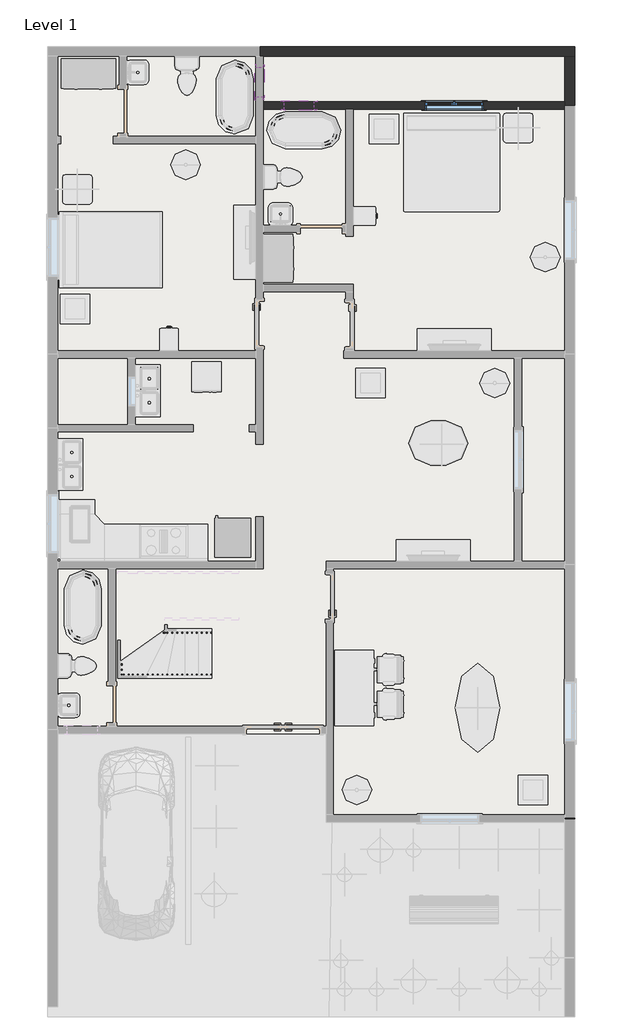
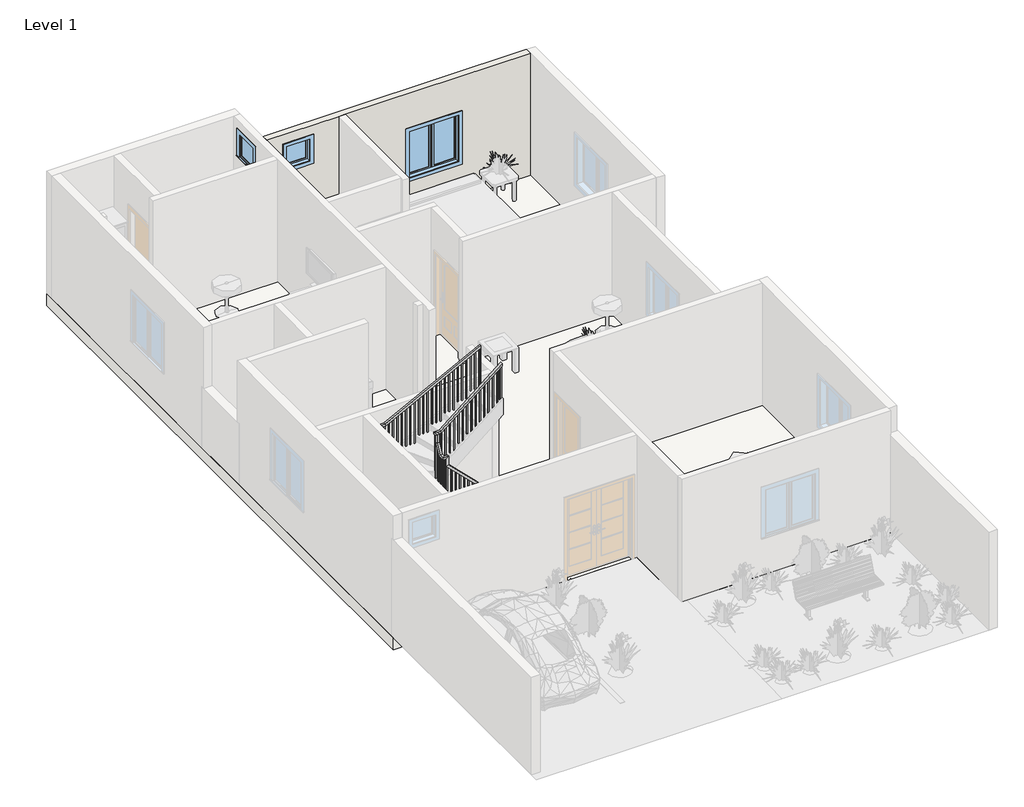
# One storey, part 2 of 3: 3 walls, 3 windows, 2 railings, 1 slab.
"""IFC4 building model written with IfcOpenShell, lengths in millimetres."""

from ifc_helpers import new_model, si_unit, frame, origin, place, context, project, spatial, polyline, outline, extrude, faceted_brep, transform, mapped, element, save
from components import window_be30da88, window_3d781103

model = new_model("IFC4")

# Units and contexts
model_context = context("Model", 3, world=origin())
ifc_project = project(units=[si_unit("LENGTHUNIT", "METRE", prefix="MILLI")], contexts=[model_context])

# Site, building, storey
site = spatial("IfcSite", under=ifc_project)
building = spatial("IfcBuilding", under=site)
storey = spatial("IfcBuildingStorey", under=building, Name="Level 1", Elevation=0.0)

# Railings
placement = place(None, origin())
element("IfcRailing", 1, ObjectType="Handrail - Rectangular", at=placement, inside=storey, context=model_context, shape_type="SolidModel", body=[
    faceted_brep([(-8420.1659688, 2032.699435, 1316.3704569), (-8420.1659688, 2032.699435, 1245.0455517), (-8420.1659688, 2083.499435, 1245.0455517), (-8420.1659688, 2083.499435, 1316.3704569), (-9312.8976606, 2032.699435, 2196.2028354), (-9363.6976606, 2032.699435, 2174.9439077), (-9363.6976606, 2083.499435, 2174.9439077), (-9312.8976606, 2083.499435, 2196.2028354), (-9312.8976606, 2032.699435, 2414.6281882), (-9363.6976606, 2032.699435, 2363.8281882), (-9363.6976606, 2083.499435, 2363.8281882), (-9312.8976606, 2083.499435, 2414.6281882), (-9439.8976606, 2032.699435, 2414.6281882), (-9439.8976606, 2032.699435, 2363.8281882), (-9389.0976606, 2083.499435, 2363.8281882), (-9389.0976606, 2083.499435, 2414.6281882), (-9439.8976606, 2159.699435, 2414.6281882), (-9439.8976606, 2188.8207688, 2363.8281882), (-9389.0976606, 2188.8207688, 2363.8281882), (-9389.0976606, 2159.699435, 2414.6281882), (-9439.8976606, 2286.699435, 2631.5051451), (-9439.8976606, 2337.499435, 2617.7256424), (-9389.0976606, 2337.499435, 2617.7256424), (-9389.0976606, 2286.699435, 2631.5051451), (-9439.8976606, 2286.699435, 2837.3484995), (-9439.8976606, 2337.499435, 2786.5484995), (-9389.0976606, 2337.499435, 2786.5484995), (-9389.0976606, 2286.699435, 2837.3484995), (-9439.8976606, 2413.699435, 2837.3484995), (-9439.8976606, 2413.699435, 2786.5484995), (-9389.0976606, 2362.899435, 2786.5484995), (-9389.0976606, 2362.899435, 2837.3484995), (-9312.8976606, 2413.699435, 2837.3484995), (-9294.8122476, 2413.699435, 2786.5484995), (-9294.8122476, 2362.899435, 2786.5484995), (-9312.8976606, 2362.899435, 2837.3484995), (-7861.3659688, 2413.699435, 4020.8803652), (-7861.3659688, 2362.899435, 4020.8803652), (-7861.3659688, 2362.899435, 3955.3341059), (-7861.3659688, 2413.699435, 3955.3341059)], [[[0, 1, 2, 3]], [[1, 0, 4, 5]], [[2, 1, 5, 6]], [[3, 2, 6, 7]], [[0, 3, 7, 4]], [[5, 4, 8, 9]], [[6, 5, 9, 10]], [[7, 6, 10, 11]], [[4, 7, 11, 8]], [[9, 8, 12, 13]], [[10, 9, 13, 14]], [[11, 10, 14, 15]], [[8, 11, 15, 12]], [[13, 12, 16, 17]], [[14, 13, 17, 18]], [[15, 14, 18, 19]], [[12, 15, 19, 16]], [[17, 16, 20, 21]], [[18, 17, 21, 22]], [[19, 18, 22, 23]], [[16, 19, 23, 20]], [[21, 20, 24, 25]], [[22, 21, 25, 26]], [[23, 22, 26, 27]], [[20, 23, 27, 24]], [[25, 24, 28, 29]], [[26, 25, 29, 30]], [[27, 26, 30, 31]], [[24, 27, 31, 28]], [[29, 28, 32, 33]], [[30, 29, 33, 34]], [[31, 30, 34, 35]], [[28, 31, 35, 32]], [[36, 37, 38, 39]], [[33, 32, 36, 39]], [[34, 33, 39, 38]], [[35, 34, 38, 37]], [[32, 35, 37, 36]]]),
    extrude(outline(polyline([(3881.7558784, -7951.6053043), (3866.2231262, -7970.6553043), (2878.6666667, -7970.6553043), (2878.6666667, -7951.6053043), (3881.7558784, -7951.6053043)])), frame((0.0, 2378.774435, 0.0), z_axis=(0.0, 1.0, 0.0), x_axis=(0.0, 0.0, 1.0)), (0.0, 0.0, 1.0), 19.05),
    extrude(outline(polyline([(3798.9145334, -8053.2053043), (3783.3817813, -8072.2553043), (2878.6666667, -8072.2553043), (2878.6666667, -8053.2053043), (3798.9145334, -8053.2053043)])), frame((0.0, 2378.774435, 0.0), z_axis=(0.0, 1.0, 0.0), x_axis=(0.0, 0.0, 1.0)), (0.0, 0.0, 1.0), 19.05),
    extrude(outline(polyline([(3716.0731885, -8154.8053043), (3700.5404364, -8173.8553043), (2709.3333333, -8173.8553043), (2709.3333333, -8154.8053043), (3716.0731885, -8154.8053043)])), frame((0.0, 2378.774435, 0.0), z_axis=(0.0, 1.0, 0.0), x_axis=(0.0, 0.0, 1.0)), (0.0, 0.0, 1.0), 19.05),
    extrude(outline(polyline([(3633.2318436, -8256.4053043), (3617.6990914, -8275.4553043), (2709.3333333, -8275.4553043), (2709.3333333, -8256.4053043), (3633.2318436, -8256.4053043)])), frame((0.0, 2378.774435, 0.0), z_axis=(0.0, 1.0, 0.0), x_axis=(0.0, 0.0, 1.0)), (0.0, 0.0, 1.0), 19.05),
    extrude(outline(polyline([(3550.3904987, -8358.0053043), (3534.8577465, -8377.0553043), (2709.3333333, -8377.0553043), (2709.3333333, -8358.0053043), (3550.3904987, -8358.0053043)])), frame((0.0, 2378.774435, 0.0), z_axis=(0.0, 1.0, 0.0), x_axis=(0.0, 0.0, 1.0)), (0.0, 0.0, 1.0), 19.05),
    extrude(outline(polyline([(3467.5491538, -8459.6053043), (3452.0164016, -8478.6553043), (2540.0, -8478.6553043), (2540.0, -8459.6053043), (3467.5491538, -8459.6053043)])), frame((0.0, 2378.774435, 0.0), z_axis=(0.0, 1.0, 0.0), x_axis=(0.0, 0.0, 1.0)), (0.0, 0.0, 1.0), 19.05),
    extrude(outline(polyline([(3384.7078088, -8561.2053043), (3369.1750567, -8580.2553043), (2540.0, -8580.2553043), (2540.0, -8561.2053043), (3384.7078088, -8561.2053043)])), frame((0.0, 2378.774435, 0.0), z_axis=(0.0, 1.0, 0.0), x_axis=(0.0, 0.0, 1.0)), (0.0, 0.0, 1.0), 19.05),
    extrude(outline(polyline([(3301.8664639, -8662.8053043), (3286.3337117, -8681.8553043), (2540.0, -8681.8553043), (2540.0, -8662.8053043), (3301.8664639, -8662.8053043)])), frame((0.0, 2378.774435, 0.0), z_axis=(0.0, 1.0, 0.0), x_axis=(0.0, 0.0, 1.0)), (0.0, 0.0, 1.0), 19.05),
    extrude(outline(polyline([(3219.025119, -8764.4053043), (3203.4923668, -8783.4553043), (2370.6666667, -8783.4553043), (2370.6666667, -8764.4053043), (3219.025119, -8764.4053043)])), frame((0.0, 2378.774435, 0.0), z_axis=(0.0, 1.0, 0.0), x_axis=(0.0, 0.0, 1.0)), (0.0, 0.0, 1.0), 19.05),
    extrude(outline(polyline([(3136.1837741, -8866.0053043), (3120.6510219, -8885.0553043), (2370.6666667, -8885.0553043), (2370.6666667, -8866.0053043), (3136.1837741, -8866.0053043)])), frame((0.0, 2378.774435, 0.0), z_axis=(0.0, 1.0, 0.0), x_axis=(0.0, 0.0, 1.0)), (0.0, 0.0, 1.0), 19.05),
    extrude(outline(polyline([(3053.3424291, -8967.6053043), (3037.809677, -8986.6553043), (2201.3333333, -8986.6553043), (2201.3333333, -8967.6053043), (3053.3424291, -8967.6053043)])), frame((0.0, 2378.774435, 0.0), z_axis=(0.0, 1.0, 0.0), x_axis=(0.0, 0.0, 1.0)), (0.0, 0.0, 1.0), 19.05),
    extrude(outline(polyline([(2970.5010842, -9069.2053043), (2954.9683321, -9088.2553043), (2201.3333333, -9088.2553043), (2201.3333333, -9069.2053043), (2970.5010842, -9069.2053043)])), frame((0.0, 2378.774435, 0.0), z_axis=(0.0, 1.0, 0.0), x_axis=(0.0, 0.0, 1.0)), (0.0, 0.0, 1.0), 19.05),
    extrude(outline(polyline([(2887.6597393, -9170.8053043), (2872.1269871, -9189.8553043), (2032.0, -9189.8553043), (2032.0, -9170.8053043), (2887.6597393, -9170.8053043)])), frame((0.0, 2378.774435, 0.0), z_axis=(0.0, 1.0, 0.0), x_axis=(0.0, 0.0, 1.0)), (0.0, 0.0, 1.0), 19.05),
    extrude(outline(polyline([(2804.8183944, -9272.4053043), (2789.2856422, -9291.4553043), (2032.0, -9291.4553043), (2032.0, -9272.4053043), (2804.8183944, -9272.4053043)])), frame((0.0, 2378.774435, 0.0), z_axis=(0.0, 1.0, 0.0), x_axis=(0.0, 0.0, 1.0)), (0.0, 0.0, 1.0), 19.05),
    extrude(outline(polyline([(2267.9389861, 2498.9377803), (2286.9889861, 2531.4693239), (2286.9889861, 1524.0), (2267.9389861, 1524.0), (2267.9389861, 2498.9377803)])), frame((-9424.0226606, 0.0, 0.0), z_axis=(1.0, 0.0, 0.0), x_axis=(0.0, 1.0, 0.0)), (0.0, 0.0, 1.0), 19.05),
    extrude(outline(polyline([(2166.3389861, 2325.4362148), (2185.3889861, 2357.9677583), (2185.3889861, 1524.0), (2166.3389861, 1524.0), (2166.3389861, 2325.4362148)])), frame((-9424.0226606, 0.0, 0.0), z_axis=(1.0, 0.0, 0.0), x_axis=(0.0, 1.0, 0.0)), (0.0, 0.0, 1.0), 19.05),
    extrude(outline(polyline([(2136.8457765, -9325.0409688), (2155.620518, -9344.0909688), (1185.3333333, -9344.0909688), (1185.3333333, -9325.0409688), (2136.8457765, -9325.0409688)])), frame((0.0, 2048.574435, 0.0), z_axis=(0.0, 1.0, 0.0), x_axis=(0.0, 0.0, 1.0)), (0.0, 0.0, 1.0), 19.05),
    extrude(outline(polyline([(2036.7138214, -9223.4409688), (2055.488563, -9242.4909688), (1016.0, -9242.4909688), (1016.0, -9223.4409688), (2036.7138214, -9223.4409688)])), frame((0.0, 2048.574435, 0.0), z_axis=(0.0, 1.0, 0.0), x_axis=(0.0, 0.0, 1.0)), (0.0, 0.0, 1.0), 19.05),
    extrude(outline(polyline([(1936.5818663, -9121.8409688), (1955.3566079, -9140.8909688), (846.6666667, -9140.8909688), (846.6666667, -9121.8409688), (1936.5818663, -9121.8409688)])), frame((0.0, 2048.574435, 0.0), z_axis=(0.0, 1.0, 0.0), x_axis=(0.0, 0.0, 1.0)), (0.0, 0.0, 1.0), 19.05),
    extrude(outline(polyline([(1836.4499113, -9020.2409688), (1855.2246528, -9039.2909688), (846.6666667, -9039.2909688), (846.6666667, -9020.2409688), (1836.4499113, -9020.2409688)])), frame((0.0, 2048.574435, 0.0), z_axis=(0.0, 1.0, 0.0), x_axis=(0.0, 0.0, 1.0)), (0.0, 0.0, 1.0), 19.05),
    extrude(outline(polyline([(1736.3179562, -8918.6409688), (1755.0926978, -8937.6909688), (677.3333333, -8937.6909688), (677.3333333, -8918.6409688), (1736.3179562, -8918.6409688)])), frame((0.0, 2048.574435, 0.0), z_axis=(0.0, 1.0, 0.0), x_axis=(0.0, 0.0, 1.0)), (0.0, 0.0, 1.0), 19.05),
    extrude(outline(polyline([(1636.1860011, -8817.0409688), (1654.9607427, -8836.0909688), (677.3333333, -8836.0909688), (677.3333333, -8817.0409688), (1636.1860011, -8817.0409688)])), frame((0.0, 2048.574435, 0.0), z_axis=(0.0, 1.0, 0.0), x_axis=(0.0, 0.0, 1.0)), (0.0, 0.0, 1.0), 19.05),
    extrude(outline(polyline([(1536.0540461, -8715.4409688), (1554.8287877, -8734.4909688), (677.3333333, -8734.4909688), (677.3333333, -8715.4409688), (1536.0540461, -8715.4409688)])), frame((0.0, 2048.574435, 0.0), z_axis=(0.0, 1.0, 0.0), x_axis=(0.0, 0.0, 1.0)), (0.0, 0.0, 1.0), 19.05),
    extrude(outline(polyline([(1435.922091, -8613.8409688), (1454.6968326, -8632.8909688), (508.0, -8632.8909688), (508.0, -8613.8409688), (1435.922091, -8613.8409688)])), frame((0.0, 2048.574435, 0.0), z_axis=(0.0, 1.0, 0.0), x_axis=(0.0, 0.0, 1.0)), (0.0, 0.0, 1.0), 19.05),
    extrude(outline(polyline([(1335.790136, -8512.2409688), (1354.5648775, -8531.2909688), (508.0, -8531.2909688), (508.0, -8512.2409688), (1335.790136, -8512.2409688)])), frame((0.0, 2048.574435, 0.0), z_axis=(0.0, 1.0, 0.0), x_axis=(0.0, 0.0, 1.0)), (0.0, 0.0, 1.0), 19.05),
    extrude(outline(polyline([(-9393.0553043, 2378.774435), (-9393.0553043, 2397.824435), (-9374.0053043, 2397.824435), (-9374.0053043, 2378.774435), (-9393.0553043, 2378.774435)])), frame((0.0, 0.0, 1862.6666667), z_axis=(0.0, 0.0, 1.0), x_axis=(1.0, 0.0, 0.0)), (0.0, 0.0, 1.0), 923.8818329),
    extrude(outline(polyline([(-9404.9726606, 2378.774435), (-9424.0226606, 2378.774435), (-9424.0226606, 2397.824435), (-9404.9726606, 2397.824435), (-9404.9726606, 2378.774435)])), frame((0.0, 0.0, 1862.6666667), z_axis=(0.0, 0.0, 1.0), x_axis=(1.0, 0.0, 0.0)), (0.0, 0.0, 1.0), 923.8818329),
    extrude(outline(polyline([(-9404.9726606, 2363.9885312), (-9424.0226606, 2363.9885312), (-9424.0226606, 2383.0385312), (-9404.9726606, 2383.0385312), (-9404.9726606, 2363.9885312)])), frame((0.0, 0.0, 1693.3333333), z_axis=(0.0, 0.0, 1.0), x_axis=(1.0, 0.0, 0.0)), (0.0, 0.0, 1.0), 1093.2151662),
    extrude(outline(polyline([(-9404.9726606, 2064.7389861), (-9424.0226606, 2064.7389861), (-9424.0226606, 2083.7889861), (-9404.9726606, 2083.7889861), (-9404.9726606, 2064.7389861)])), frame((0.0, 0.0, 1354.6666667), z_axis=(0.0, 0.0, 1.0), x_axis=(1.0, 0.0, 0.0)), (0.0, 0.0, 1.0), 1009.1615215),
    extrude(outline(polyline([(-9404.9726606, 2067.624435), (-9404.9726606, 2048.574435), (-9424.0226606, 2048.574435), (-9424.0226606, 2067.624435), (-9404.9726606, 2067.624435)])), frame((0.0, 0.0, 1185.3333333), z_axis=(0.0, 0.0, 1.0), x_axis=(1.0, 0.0, 0.0)), (0.0, 0.0, 1.0), 1178.4948549),
    extrude(outline(polyline([(-9376.9638704, 2067.624435), (-9376.9638704, 2048.574435), (-9396.0138704, 2048.574435), (-9396.0138704, 2067.624435), (-9376.9638704, 2067.624435)])), frame((0.0, 0.0, 1185.3333333), z_axis=(0.0, 0.0, 1.0), x_axis=(1.0, 0.0, 0.0)), (0.0, 0.0, 1.0), 1178.4948549),
    extrude(outline(polyline([(3955.3341059, -7861.3659688), (3939.8013537, -7880.4159688), (2878.6666667, -7880.4159688), (2878.6666667, -7861.3659688), (3955.3341059, -7861.3659688)])), frame((0.0, 2378.774435, 0.0), z_axis=(0.0, 1.0, 0.0), x_axis=(0.0, 0.0, 1.0)), (0.0, 0.0, 1.0), 19.05),
    extrude(outline(polyline([(1245.0455517, -8420.1659688), (1263.8202933, -8439.2159688), (508.0, -8439.2159688), (508.0, -8420.1659688), (1245.0455517, -8420.1659688)])), frame((0.0, 2048.574435, 0.0), z_axis=(0.0, 1.0, 0.0), x_axis=(0.0, 0.0, 1.0)), (0.0, 0.0, 1.0), 19.05),
])
element("IfcRailing", 2, ObjectType="Handrail - Rectangular", at=placement, inside=storey, context=model_context, shape_type="SolidModel", body=[
    faceted_brep([(-8420.1659688, 1169.099435, 1460.80748), (-8420.1659688, 1169.099435, 1404.7066442), (-8420.1659688, 1219.899435, 1404.7066442), (-8420.1659688, 1219.899435, 1460.80748), (-10130.375003, 1169.099435, 2262.2053941), (-10141.6871577, 1169.099435, 2211.4053941), (-10141.6871577, 1219.899435, 2211.4053941), (-10130.375003, 1219.899435, 2262.2053941), (-10303.4976606, 1169.099435, 2262.2053941), (-10303.4976606, 1169.099435, 2211.4053941), (-10252.6976606, 1219.899435, 2211.4053941), (-10252.6976606, 1219.899435, 2262.2053941), (-10303.4976606, 1410.2296279, 2262.2053941), (-10303.4976606, 1418.180204, 2211.4053941), (-10252.6976606, 1418.180204, 2211.4053941), (-10252.6976606, 1410.2296279, 2262.2053941), (-10303.4976606, 3000.1454824, 2772.3688337), (-10303.4976606, 3008.0960585, 2721.5688337), (-10252.6976606, 3008.0960585, 2721.5688337), (-10252.6976606, 3000.1454824, 2772.3688337), (-10303.4976606, 3277.299435, 2772.3688337), (-10303.4976606, 3277.299435, 2721.5688337), (-10252.6976606, 3226.499435, 2721.5688337), (-10252.6976606, 3226.499435, 2772.3688337), (-10121.3478253, 3277.299435, 2772.3688337), (-10109.027774, 3277.299435, 2721.5688337), (-10109.027774, 3226.499435, 2721.5688337), (-10121.3478253, 3226.499435, 2772.3688337), (-7861.3659688, 3277.299435, 3937.0561582), (-7861.3659688, 3226.499435, 3937.0561582), (-7861.3659688, 3226.499435, 3879.9069889), (-7861.3659688, 3277.299435, 3879.9069889)], [[[0, 1, 2, 3]], [[1, 0, 4, 5]], [[2, 1, 5, 6]], [[3, 2, 6, 7]], [[0, 3, 7, 4]], [[5, 4, 8, 9]], [[6, 5, 9, 10]], [[7, 6, 10, 11]], [[4, 7, 11, 8]], [[9, 8, 12, 13]], [[10, 9, 13, 14]], [[11, 10, 14, 15]], [[8, 11, 15, 12]], [[13, 12, 16, 17]], [[14, 13, 17, 18]], [[15, 14, 18, 19]], [[12, 15, 19, 16]], [[17, 16, 20, 21]], [[18, 17, 21, 22]], [[19, 18, 22, 23]], [[16, 19, 23, 20]], [[21, 20, 24, 25]], [[22, 21, 25, 26]], [[23, 22, 26, 27]], [[20, 23, 27, 24]], [[28, 29, 30, 31]], [[25, 24, 28, 31]], [[26, 25, 31, 30]], [[27, 26, 30, 29]], [[24, 27, 29, 28]]]),
    extrude(outline(polyline([(3862.2268642, -7895.6728253), (2878.6666667, -7895.6728253), (2878.6666667, -7876.6228253), (3872.0443296, -7876.6228253), (3862.2268642, -7895.6728253)])), frame((0.0, 3242.374435, 0.0), z_axis=(0.0, 1.0, 0.0), x_axis=(0.0, 0.0, 1.0)), (0.0, 0.0, 1.0), 19.05),
    extrude(outline(polyline([(3809.8670491, -7997.2728253), (2878.6666667, -7997.2728253), (2878.6666667, -7978.2228253), (3819.6845145, -7978.2228253), (3809.8670491, -7997.2728253)])), frame((0.0, 3242.374435, 0.0), z_axis=(0.0, 1.0, 0.0), x_axis=(0.0, 0.0, 1.0)), (0.0, 0.0, 1.0), 19.05),
    extrude(outline(polyline([(3757.507234, -8098.8728253), (2878.6666667, -8098.8728253), (2878.6666667, -8079.8228253), (3767.3246993, -8079.8228253), (3757.507234, -8098.8728253)])), frame((0.0, 3242.374435, 0.0), z_axis=(0.0, 1.0, 0.0), x_axis=(0.0, 0.0, 1.0)), (0.0, 0.0, 1.0), 19.05),
    extrude(outline(polyline([(3705.1474189, -8200.4728253), (2709.3333333, -8200.4728253), (2709.3333333, -8181.4228253), (3714.9648842, -8181.4228253), (3705.1474189, -8200.4728253)])), frame((0.0, 3242.374435, 0.0), z_axis=(0.0, 1.0, 0.0), x_axis=(0.0, 0.0, 1.0)), (0.0, 0.0, 1.0), 19.05),
    extrude(outline(polyline([(3652.7876038, -8302.0728253), (2709.3333333, -8302.0728253), (2709.3333333, -8283.0228253), (3662.6050691, -8283.0228253), (3652.7876038, -8302.0728253)])), frame((0.0, 3242.374435, 0.0), z_axis=(0.0, 1.0, 0.0), x_axis=(0.0, 0.0, 1.0)), (0.0, 0.0, 1.0), 19.05),
    extrude(outline(polyline([(3600.4277887, -8403.6728253), (2709.3333333, -8403.6728253), (2709.3333333, -8384.6228253), (3610.245254, -8384.6228253), (3600.4277887, -8403.6728253)])), frame((0.0, 3242.374435, 0.0), z_axis=(0.0, 1.0, 0.0), x_axis=(0.0, 0.0, 1.0)), (0.0, 0.0, 1.0), 19.05),
    extrude(outline(polyline([(3548.0679735, -8505.2728253), (2540.0, -8505.2728253), (2540.0, -8486.2228253), (3557.8854389, -8486.2228253), (3548.0679735, -8505.2728253)])), frame((0.0, 3242.374435, 0.0), z_axis=(0.0, 1.0, 0.0), x_axis=(0.0, 0.0, 1.0)), (0.0, 0.0, 1.0), 19.05),
    extrude(outline(polyline([(3495.7081584, -8606.8728253), (2540.0, -8606.8728253), (2540.0, -8587.8228253), (3505.5256238, -8587.8228253), (3495.7081584, -8606.8728253)])), frame((0.0, 3242.374435, 0.0), z_axis=(0.0, 1.0, 0.0), x_axis=(0.0, 0.0, 1.0)), (0.0, 0.0, 1.0), 19.05),
    extrude(outline(polyline([(3443.3483433, -8708.4728253), (2540.0, -8708.4728253), (2540.0, -8689.4228253), (3453.1658086, -8689.4228253), (3443.3483433, -8708.4728253)])), frame((0.0, 3242.374435, 0.0), z_axis=(0.0, 1.0, 0.0), x_axis=(0.0, 0.0, 1.0)), (0.0, 0.0, 1.0), 19.05),
    extrude(outline(polyline([(3390.9885282, -8810.0728253), (2370.6666667, -8810.0728253), (2370.6666667, -8791.0228253), (3400.8059935, -8791.0228253), (3390.9885282, -8810.0728253)])), frame((0.0, 3242.374435, 0.0), z_axis=(0.0, 1.0, 0.0), x_axis=(0.0, 0.0, 1.0)), (0.0, 0.0, 1.0), 19.05),
    extrude(outline(polyline([(3338.6287131, -8911.6728253), (2370.6666667, -8911.6728253), (2370.6666667, -8892.6228253), (3348.4461784, -8892.6228253), (3338.6287131, -8911.6728253)])), frame((0.0, 3242.374435, 0.0), z_axis=(0.0, 1.0, 0.0), x_axis=(0.0, 0.0, 1.0)), (0.0, 0.0, 1.0), 19.05),
    extrude(outline(polyline([(3286.268898, -9013.2728253), (2370.6666667, -9013.2728253), (2370.6666667, -8994.2228253), (3296.0863633, -8994.2228253), (3286.268898, -9013.2728253)])), frame((0.0, 3242.374435, 0.0), z_axis=(0.0, 1.0, 0.0), x_axis=(0.0, 0.0, 1.0)), (0.0, 0.0, 1.0), 19.05),
    extrude(outline(polyline([(3233.9090828, -9114.8728253), (2201.3333333, -9114.8728253), (2201.3333333, -9095.8228253), (3243.7265482, -9095.8228253), (3233.9090828, -9114.8728253)])), frame((0.0, 3242.374435, 0.0), z_axis=(0.0, 1.0, 0.0), x_axis=(0.0, 0.0, 1.0)), (0.0, 0.0, 1.0), 19.05),
    extrude(outline(polyline([(3181.5492677, -9216.4728253), (2201.3333333, -9216.4728253), (2201.3333333, -9197.4228253), (3191.3667331, -9197.4228253), (3181.5492677, -9216.4728253)])), frame((0.0, 3242.374435, 0.0), z_axis=(0.0, 1.0, 0.0), x_axis=(0.0, 0.0, 1.0)), (0.0, 0.0, 1.0), 19.05),
    extrude(outline(polyline([(3129.1894526, -9318.0728253), (2201.3333333, -9318.0728253), (2201.3333333, -9299.0228253), (3139.0069179, -9299.0228253), (3129.1894526, -9318.0728253)])), frame((0.0, 3242.374435, 0.0), z_axis=(0.0, 1.0, 0.0), x_axis=(0.0, 0.0, 1.0)), (0.0, 0.0, 1.0), 19.05),
    extrude(outline(polyline([(3076.8296375, -9419.6728253), (2032.0, -9419.6728253), (2032.0, -9400.6228253), (3086.6471028, -9400.6228253), (3076.8296375, -9419.6728253)])), frame((0.0, 3242.374435, 0.0), z_axis=(0.0, 1.0, 0.0), x_axis=(0.0, 0.0, 1.0)), (0.0, 0.0, 1.0), 19.05),
    extrude(outline(polyline([(3024.4698224, -9521.2728253), (2032.0, -9521.2728253), (2032.0, -9502.2228253), (3034.2872877, -9502.2228253), (3024.4698224, -9521.2728253)])), frame((0.0, 3242.374435, 0.0), z_axis=(0.0, 1.0, 0.0), x_axis=(0.0, 0.0, 1.0)), (0.0, 0.0, 1.0), 19.05),
    extrude(outline(polyline([(2972.1100073, -9622.8728253), (2032.0, -9622.8728253), (2032.0, -9603.8228253), (2981.9274726, -9603.8228253), (2972.1100073, -9622.8728253)])), frame((0.0, 3242.374435, 0.0), z_axis=(0.0, 1.0, 0.0), x_axis=(0.0, 0.0, 1.0)), (0.0, 0.0, 1.0), 19.05),
    extrude(outline(polyline([(2919.7501921, -9724.4728253), (2032.0, -9724.4728253), (2032.0, -9705.4228253), (2929.5676575, -9705.4228253), (2919.7501921, -9724.4728253)])), frame((0.0, 3242.374435, 0.0), z_axis=(0.0, 1.0, 0.0), x_axis=(0.0, 0.0, 1.0)), (0.0, 0.0, 1.0), 19.05),
    extrude(outline(polyline([(2867.390377, -9826.0728253), (1862.6666667, -9826.0728253), (1862.6666667, -9807.0228253), (2877.2078424, -9807.0228253), (2867.390377, -9826.0728253)])), frame((0.0, 3242.374435, 0.0), z_axis=(0.0, 1.0, 0.0), x_axis=(0.0, 0.0, 1.0)), (0.0, 0.0, 1.0), 19.05),
    extrude(outline(polyline([(2815.0305619, -9927.6728253), (1862.6666667, -9927.6728253), (1862.6666667, -9908.6228253), (2824.8480272, -9908.6228253), (2815.0305619, -9927.6728253)])), frame((0.0, 3242.374435, 0.0), z_axis=(0.0, 1.0, 0.0), x_axis=(0.0, 0.0, 1.0)), (0.0, 0.0, 1.0), 19.05),
    extrude(outline(polyline([(2762.6707468, -10029.2728253), (1862.6666667, -10029.2728253), (1862.6666667, -10010.2228253), (2772.4882121, -10010.2228253), (2762.6707468, -10029.2728253)])), frame((0.0, 3242.374435, 0.0), z_axis=(0.0, 1.0, 0.0), x_axis=(0.0, 0.0, 1.0)), (0.0, 0.0, 1.0), 19.05),
    extrude(outline(polyline([(-10186.0226606, 3261.424435), (-10166.9726606, 3261.424435), (-10166.9726606, 3242.374435), (-10186.0226606, 3242.374435), (-10186.0226606, 3261.424435)])), frame((0.0, 0.0, 1862.6666667), z_axis=(0.0, 0.0, 1.0), x_axis=(1.0, 0.0, 0.0)), (0.0, 0.0, 1.0), 858.902167),
    extrude(outline(polyline([(-10287.6226606, 3193.8204824), (-10287.6226606, 3212.8704824), (-10268.5726606, 3212.8704824), (-10268.5726606, 3193.8204824), (-10287.6226606, 3193.8204824)])), frame((0.0, 0.0, 1862.6666667), z_axis=(0.0, 0.0, 1.0), x_axis=(1.0, 0.0, 0.0)), (0.0, 0.0, 1.0), 858.902167),
    extrude(outline(polyline([(-10287.6226606, 3092.2204824), (-10287.6226606, 3111.2704824), (-10268.5726606, 3111.2704824), (-10268.5726606, 3092.2204824), (-10287.6226606, 3092.2204824)])), frame((0.0, 0.0, 1862.6666667), z_axis=(0.0, 0.0, 1.0), x_axis=(1.0, 0.0, 0.0)), (0.0, 0.0, 1.0), 858.902167),
    extrude(outline(polyline([(2943.7546279, 2700.9233099), (2943.7546279, 1693.3333333), (2924.7046279, 1693.3333333), (2924.7046279, 2694.8106509), (2943.7546279, 2700.9233099)])), frame((-10287.6226606, 0.0, 0.0), z_axis=(1.0, 0.0, 0.0), x_axis=(0.0, 1.0, 0.0)), (0.0, 0.0, 1.0), 19.05),
    extrude(outline(polyline([(2842.1546279, 2668.3224617), (2842.1546279, 1693.3333333), (2823.1046279, 1693.3333333), (2823.1046279, 2662.2098027), (2842.1546279, 2668.3224617)])), frame((-10287.6226606, 0.0, 0.0), z_axis=(1.0, 0.0, 0.0), x_axis=(0.0, 1.0, 0.0)), (0.0, 0.0, 1.0), 19.05),
    extrude(outline(polyline([(2740.5546279, 2635.7216135), (2740.5546279, 1693.3333333), (2721.5046279, 1693.3333333), (2721.5046279, 2629.6089544), (2740.5546279, 2635.7216135)])), frame((-10287.6226606, 0.0, 0.0), z_axis=(1.0, 0.0, 0.0), x_axis=(0.0, 1.0, 0.0)), (0.0, 0.0, 1.0), 19.05),
    extrude(outline(polyline([(2638.9546279, 2603.1207653), (2638.9546279, 1693.3333333), (2619.9046279, 1693.3333333), (2619.9046279, 2597.0081062), (2638.9546279, 2603.1207653)])), frame((-10287.6226606, 0.0, 0.0), z_axis=(1.0, 0.0, 0.0), x_axis=(0.0, 1.0, 0.0)), (0.0, 0.0, 1.0), 19.05),
    extrude(outline(polyline([(2537.3546279, 2570.519917), (2537.3546279, 1693.3333333), (2518.3046279, 1693.3333333), (2518.3046279, 2564.407258), (2537.3546279, 2570.519917)])), frame((-10287.6226606, 0.0, 0.0), z_axis=(1.0, 0.0, 0.0), x_axis=(0.0, 1.0, 0.0)), (0.0, 0.0, 1.0), 19.05),
    extrude(outline(polyline([(2435.7546279, 2537.9190688), (2435.7546279, 1524.0), (2416.7046279, 1524.0), (2416.7046279, 2531.8064098), (2435.7546279, 2537.9190688)])), frame((-10287.6226606, 0.0, 0.0), z_axis=(1.0, 0.0, 0.0), x_axis=(0.0, 1.0, 0.0)), (0.0, 0.0, 1.0), 19.05),
    extrude(outline(polyline([(2334.1546279, 2505.3182206), (2334.1546279, 1524.0), (2315.1046279, 1524.0), (2315.1046279, 2499.2055615), (2334.1546279, 2505.3182206)])), frame((-10287.6226606, 0.0, 0.0), z_axis=(1.0, 0.0, 0.0), x_axis=(0.0, 1.0, 0.0)), (0.0, 0.0, 1.0), 19.05),
    extrude(outline(polyline([(2232.5546279, 2472.7173724), (2232.5546279, 1524.0), (2213.5046279, 1524.0), (2213.5046279, 2466.6047133), (2232.5546279, 2472.7173724)])), frame((-10287.6226606, 0.0, 0.0), z_axis=(1.0, 0.0, 0.0), x_axis=(0.0, 1.0, 0.0)), (0.0, 0.0, 1.0), 19.05),
    extrude(outline(polyline([(2130.9546279, 2440.1165241), (2130.9546279, 1524.0), (2111.9046279, 1524.0), (2111.9046279, 2434.0038651), (2130.9546279, 2440.1165241)])), frame((-10287.6226606, 0.0, 0.0), z_axis=(1.0, 0.0, 0.0), x_axis=(0.0, 1.0, 0.0)), (0.0, 0.0, 1.0), 19.05),
    extrude(outline(polyline([(2029.3546279, 2407.5156759), (2029.3546279, 1524.0), (2010.3046279, 1524.0), (2010.3046279, 2401.4030169), (2029.3546279, 2407.5156759)])), frame((-10287.6226606, 0.0, 0.0), z_axis=(1.0, 0.0, 0.0), x_axis=(0.0, 1.0, 0.0)), (0.0, 0.0, 1.0), 19.05),
    extrude(outline(polyline([(1927.7546279, 2374.9148277), (1927.7546279, 1354.6666667), (1908.7046279, 1354.6666667), (1908.7046279, 2368.8021686), (1927.7546279, 2374.9148277)])), frame((-10287.6226606, 0.0, 0.0), z_axis=(1.0, 0.0, 0.0), x_axis=(0.0, 1.0, 0.0)), (0.0, 0.0, 1.0), 19.05),
    extrude(outline(polyline([(1826.1546279, 2342.3139794), (1826.1546279, 1354.6666667), (1807.1046279, 1354.6666667), (1807.1046279, 2336.2013204), (1826.1546279, 2342.3139794)])), frame((-10287.6226606, 0.0, 0.0), z_axis=(1.0, 0.0, 0.0), x_axis=(0.0, 1.0, 0.0)), (0.0, 0.0, 1.0), 19.05),
    extrude(outline(polyline([(1724.5546279, 2309.7131312), (1724.5546279, 1354.6666667), (1705.5046279, 1354.6666667), (1705.5046279, 2303.6004722), (1724.5546279, 2309.7131312)])), frame((-10287.6226606, 0.0, 0.0), z_axis=(1.0, 0.0, 0.0), x_axis=(0.0, 1.0, 0.0)), (0.0, 0.0, 1.0), 19.05),
    extrude(outline(polyline([(1622.9546279, 2277.112283), (1622.9546279, 1354.6666667), (1603.9046279, 1354.6666667), (1603.9046279, 2270.999624), (1622.9546279, 2277.112283)])), frame((-10287.6226606, 0.0, 0.0), z_axis=(1.0, 0.0, 0.0), x_axis=(0.0, 1.0, 0.0)), (0.0, 0.0, 1.0), 19.05),
    extrude(outline(polyline([(1521.3546279, 2244.5114348), (1521.3546279, 1354.6666667), (1502.3046279, 1354.6666667), (1502.3046279, 2238.3987757), (1521.3546279, 2244.5114348)])), frame((-10287.6226606, 0.0, 0.0), z_axis=(1.0, 0.0, 0.0), x_axis=(0.0, 1.0, 0.0)), (0.0, 0.0, 1.0), 19.05),
    extrude(outline(polyline([(-10287.6226606, 1388.174435), (-10287.6226606, 1407.224435), (-10268.5726606, 1407.224435), (-10268.5726606, 1388.174435), (-10287.6226606, 1388.174435)])), frame((0.0, 0.0, 1185.3333333), z_axis=(0.0, 0.0, 1.0), x_axis=(1.0, 0.0, 0.0)), (0.0, 0.0, 1.0), 1026.0720608),
    extrude(outline(polyline([(-10287.6226606, 1286.574435), (-10287.6226606, 1305.624435), (-10268.5726606, 1305.624435), (-10268.5726606, 1286.574435), (-10287.6226606, 1286.574435)])), frame((0.0, 0.0, 1185.3333333), z_axis=(0.0, 0.0, 1.0), x_axis=(1.0, 0.0, 0.0)), (0.0, 0.0, 1.0), 1026.0720608),
    extrude(outline(polyline([(-10222.450003, 1184.974435), (-10241.500003, 1184.974435), (-10241.500003, 1204.024435), (-10222.450003, 1204.024435), (-10222.450003, 1184.974435)])), frame((0.0, 0.0, 1185.3333333), z_axis=(0.0, 0.0, 1.0), x_axis=(1.0, 0.0, 0.0)), (0.0, 0.0, 1.0), 1026.0720608),
    extrude(outline(polyline([(2170.9204451, -10055.2909688), (1185.3333333, -10055.2909688), (1185.3333333, -10036.2409688), (2161.9936823, -10036.2409688), (2170.9204451, -10055.2909688)])), frame((0.0, 1184.974435, 0.0), z_axis=(0.0, 1.0, 0.0), x_axis=(0.0, 0.0, 1.0)), (0.0, 0.0, 1.0), 19.05),
    extrude(outline(polyline([(2123.3110438, -9953.6909688), (1185.3333333, -9953.6909688), (1185.3333333, -9934.6409688), (2114.3842811, -9934.6409688), (2123.3110438, -9953.6909688)])), frame((0.0, 1184.974435, 0.0), z_axis=(0.0, 1.0, 0.0), x_axis=(0.0, 0.0, 1.0)), (0.0, 0.0, 1.0), 19.05),
    extrude(outline(polyline([(2075.7016426, -9852.0909688), (1185.3333333, -9852.0909688), (1185.3333333, -9833.0409688), (2066.7748799, -9833.0409688), (2075.7016426, -9852.0909688)])), frame((0.0, 1184.974435, 0.0), z_axis=(0.0, 1.0, 0.0), x_axis=(0.0, 0.0, 1.0)), (0.0, 0.0, 1.0), 19.05),
    extrude(outline(polyline([(2028.0922414, -9750.4909688), (1016.0, -9750.4909688), (1016.0, -9731.4409688), (2019.1654787, -9731.4409688), (2028.0922414, -9750.4909688)])), frame((0.0, 1184.974435, 0.0), z_axis=(0.0, 1.0, 0.0), x_axis=(0.0, 0.0, 1.0)), (0.0, 0.0, 1.0), 19.05),
    extrude(outline(polyline([(1980.4828402, -9648.8909688), (1016.0, -9648.8909688), (1016.0, -9629.8409688), (1971.5560775, -9629.8409688), (1980.4828402, -9648.8909688)])), frame((0.0, 1184.974435, 0.0), z_axis=(0.0, 1.0, 0.0), x_axis=(0.0, 0.0, 1.0)), (0.0, 0.0, 1.0), 19.05),
    extrude(outline(polyline([(1932.873439, -9547.2909688), (1016.0, -9547.2909688), (1016.0, -9528.2409688), (1923.9466763, -9528.2409688), (1932.873439, -9547.2909688)])), frame((0.0, 1184.974435, 0.0), z_axis=(0.0, 1.0, 0.0), x_axis=(0.0, 0.0, 1.0)), (0.0, 0.0, 1.0), 19.05),
    extrude(outline(polyline([(1885.2640378, -9445.6909688), (1016.0, -9445.6909688), (1016.0, -9426.6409688), (1876.337275, -9426.6409688), (1885.2640378, -9445.6909688)])), frame((0.0, 1184.974435, 0.0), z_axis=(0.0, 1.0, 0.0), x_axis=(0.0, 0.0, 1.0)), (0.0, 0.0, 1.0), 19.05),
    extrude(outline(polyline([(1837.6546366, -9344.0909688), (846.6666667, -9344.0909688), (846.6666667, -9325.0409688), (1828.7278738, -9325.0409688), (1837.6546366, -9344.0909688)])), frame((0.0, 1184.974435, 0.0), z_axis=(0.0, 1.0, 0.0), x_axis=(0.0, 0.0, 1.0)), (0.0, 0.0, 1.0), 19.05),
    extrude(outline(polyline([(1790.0452353, -9242.4909688), (846.6666667, -9242.4909688), (846.6666667, -9223.4409688), (1781.1184726, -9223.4409688), (1790.0452353, -9242.4909688)])), frame((0.0, 1184.974435, 0.0), z_axis=(0.0, 1.0, 0.0), x_axis=(0.0, 0.0, 1.0)), (0.0, 0.0, 1.0), 19.05),
    extrude(outline(polyline([(1742.4358341, -9140.8909688), (846.6666667, -9140.8909688), (846.6666667, -9121.8409688), (1733.5090714, -9121.8409688), (1742.4358341, -9140.8909688)])), frame((0.0, 1184.974435, 0.0), z_axis=(0.0, 1.0, 0.0), x_axis=(0.0, 0.0, 1.0)), (0.0, 0.0, 1.0), 19.05),
    extrude(outline(polyline([(1694.8264329, -9039.2909688), (846.6666667, -9039.2909688), (846.6666667, -9020.2409688), (1685.8996702, -9020.2409688), (1694.8264329, -9039.2909688)])), frame((0.0, 1184.974435, 0.0), z_axis=(0.0, 1.0, 0.0), x_axis=(0.0, 0.0, 1.0)), (0.0, 0.0, 1.0), 19.05),
    extrude(outline(polyline([(1647.2170317, -8937.6909688), (677.3333333, -8937.6909688), (677.3333333, -8918.6409688), (1638.290269, -8918.6409688), (1647.2170317, -8937.6909688)])), frame((0.0, 1184.974435, 0.0), z_axis=(0.0, 1.0, 0.0), x_axis=(0.0, 0.0, 1.0)), (0.0, 0.0, 1.0), 19.05),
    extrude(outline(polyline([(1599.6076305, -8836.0909688), (677.3333333, -8836.0909688), (677.3333333, -8817.0409688), (1590.6808677, -8817.0409688), (1599.6076305, -8836.0909688)])), frame((0.0, 1184.974435, 0.0), z_axis=(0.0, 1.0, 0.0), x_axis=(0.0, 0.0, 1.0)), (0.0, 0.0, 1.0), 19.05),
    extrude(outline(polyline([(1551.9982293, -8734.4909688), (677.3333333, -8734.4909688), (677.3333333, -8715.4409688), (1543.0714665, -8715.4409688), (1551.9982293, -8734.4909688)])), frame((0.0, 1184.974435, 0.0), z_axis=(0.0, 1.0, 0.0), x_axis=(0.0, 0.0, 1.0)), (0.0, 0.0, 1.0), 19.05),
    extrude(outline(polyline([(1504.388828, -8632.8909688), (508.0, -8632.8909688), (508.0, -8613.8409688), (1495.4620653, -8613.8409688), (1504.388828, -8632.8909688)])), frame((0.0, 1184.974435, 0.0), z_axis=(0.0, 1.0, 0.0), x_axis=(0.0, 0.0, 1.0)), (0.0, 0.0, 1.0), 19.05),
    extrude(outline(polyline([(1456.7794268, -8531.2909688), (508.0, -8531.2909688), (508.0, -8512.2409688), (1447.8526641, -8512.2409688), (1456.7794268, -8531.2909688)])), frame((0.0, 1184.974435, 0.0), z_axis=(0.0, 1.0, 0.0), x_axis=(0.0, 0.0, 1.0)), (0.0, 0.0, 1.0), 19.05),
    extrude(outline(polyline([(-10130.8728253, 3261.424435), (-10111.8228253, 3261.424435), (-10111.8228253, 3242.374435), (-10130.8728253, 3242.374435), (-10130.8728253, 3261.424435)])), frame((0.0, 0.0, 1862.6666667), z_axis=(0.0, 0.0, 1.0), x_axis=(1.0, 0.0, 0.0)), (0.0, 0.0, 1.0), 858.902167),
    extrude(outline(polyline([(-10287.6226606, 3242.374435), (-10287.6226606, 3261.424435), (-10268.5726606, 3261.424435), (-10268.5726606, 3242.374435), (-10287.6226606, 3242.374435)])), frame((0.0, 0.0, 1862.6666667), z_axis=(0.0, 0.0, 1.0), x_axis=(1.0, 0.0, 0.0)), (0.0, 0.0, 1.0), 858.902167),
    extrude(outline(polyline([(3009.6704824, 2722.0740262), (3009.6704824, 1862.6666667), (2990.6204824, 1862.6666667), (2990.6204824, 2715.9613671), (3009.6704824, 2722.0740262)])), frame((-10287.6226606, 0.0, 0.0), z_axis=(1.0, 0.0, 0.0), x_axis=(0.0, 1.0, 0.0)), (0.0, 0.0, 1.0), 19.05),
    extrude(outline(polyline([(-10287.6226606, 1400.7046279), (-10287.6226606, 1419.7546279), (-10268.5726606, 1419.7546279), (-10268.5726606, 1400.7046279), (-10287.6226606, 1400.7046279)])), frame((0.0, 0.0, 1185.3333333), z_axis=(0.0, 0.0, 1.0), x_axis=(1.0, 0.0, 0.0)), (0.0, 0.0, 1.0), 1026.0720608),
    extrude(outline(polyline([(-10268.5726606, 1184.974435), (-10287.6226606, 1184.974435), (-10287.6226606, 1204.024435), (-10268.5726606, 1204.024435), (-10268.5726606, 1184.974435)])), frame((0.0, 0.0, 1185.3333333), z_axis=(0.0, 0.0, 1.0), x_axis=(1.0, 0.0, 0.0)), (0.0, 0.0, 1.0), 1026.0720608),
    extrude(outline(polyline([(2210.5679397, -10139.900003), (1185.3333333, -10139.900003), (1185.3333333, -10120.850003), (2201.641177, -10120.850003), (2210.5679397, -10139.900003)])), frame((0.0, 1184.974435, 0.0), z_axis=(0.0, 1.0, 0.0), x_axis=(0.0, 0.0, 1.0)), (0.0, 0.0, 1.0), 19.05),
    extrude(outline(polyline([(3870.0895235, -7880.4159688), (2878.6666667, -7880.4159688), (2878.6666667, -7861.3659688), (3879.9069889, -7861.3659688), (3870.0895235, -7880.4159688)])), frame((0.0, 3242.374435, 0.0), z_axis=(0.0, 1.0, 0.0), x_axis=(0.0, 0.0, 1.0)), (0.0, 0.0, 1.0), 19.05),
    extrude(outline(polyline([(1413.633407, -8439.2159688), (508.0, -8439.2159688), (508.0, -8420.1659688), (1404.7066442, -8420.1659688), (1413.633407, -8439.2159688)])), frame((0.0, 1184.974435, 0.0), z_axis=(0.0, 1.0, 0.0), x_axis=(0.0, 0.0, 1.0)), (0.0, 0.0, 1.0), 19.05),
])

# Slab
element("IfcSlab", 3, ObjectType="Generic - 12\"", at=placement, inside=storey, context=model_context, shape_type="SweptSolid", body=[
    extrude(outline(polyline([(-930.8976606, 14148.499435), (-930.8976606, -1853.500565), (-6061.6976606, -1853.500565), (-6061.6976606, -24.700565), (-11802.0976606, -24.700565), (-11802.0976606, 14148.499435), (-930.8976606, 14148.499435)])), frame((0.0, 0.0, -304.8), z_axis=(0.0, 0.0, 1.0), x_axis=(1.0, 0.0, 0.0)), (0.0, 0.0, 1.0), 304.8),
])

# Walls
element("IfcWall", 4, ObjectType="Generic - 8\"", at=placement, inside=storey, context=model_context, shape_type="Brep", body=[
    faceted_brep([(-1134.0976606, 13945.299435, 0.0), (-1134.0976606, 13005.499435, 0.0), (-1134.0976606, 12929.299435, 0.0), (-1134.0976606, 12929.299435, 1524.0), (-1134.0976606, 13005.499435, 1524.0), (-1134.0976606, 13945.299435, 1524.0), (-930.8976606, 13945.299435, 0.0), (-930.8976606, 13945.299435, 1524.0), (-930.8976606, 13005.499435, 1524.0), (-930.8976606, 12929.299435, 1524.0), (-930.8976606, 12929.299435, 0.0)], [[[0, 1, 2, 3, 4, 5]], [[6, 7, 8, 9, 10]], [[2, 1, 0, 6, 10]], [[3, 2, 10, 9]], [[5, 4, 3, 9, 8, 7]], [[0, 5, 7, 6]]]),
])
element("IfcWall", 5, ObjectType="Generic - 8\"", at=placement, inside=storey, context=model_context, shape_type="Brep", body=[
    faceted_brep([(-7433.2976606, 13945.299435, 0.0), (-7357.0976606, 13945.299435, 0.0), (-1134.0976606, 13945.299435, 0.0), (-930.8976606, 13945.299435, 0.0), (-930.8976606, 13945.299435, 1524.0), (-1134.0976606, 13945.299435, 1524.0), (-7357.0976606, 13945.299435, 1524.0), (-7433.2976606, 13945.299435, 1524.0), (-7433.2976606, 14148.499435, 0.0), (-7433.2976606, 14148.499435, 1524.0), (-7357.0976606, 14148.499435, 1524.0), (-930.8976606, 14148.499435, 1524.0), (-930.8976606, 14148.499435, 0.0)], [[[0, 1, 2, 3, 4, 5, 6, 7]], [[8, 9, 10, 11, 12]], [[3, 2, 1, 0, 8, 12]], [[7, 6, 5, 4, 11, 10, 9]], [[0, 7, 9, 8]], [[4, 3, 12, 11]]]),
])
element("IfcWall", 6, ObjectType="INNER 6\"", at=placement, inside=storey, context=model_context, shape_type="Brep", body=[
    faceted_brep([(-7357.0976606, 12853.099435, 0.0), (-5655.2976606, 12853.099435, 0.0), (-5502.8976606, 12853.099435, 0.0), (-1134.0976606, 12853.099435, 0.0), (-1134.0976606, 12853.099435, 3048.0), (-5502.8976606, 12853.099435, 3048.0), (-5655.2976606, 12853.099435, 3048.0), (-7357.0976606, 12853.099435, 3048.0), (-2810.4976606, 12853.099435, 2133.6), (-2810.4976606, 12853.099435, 914.4), (-4029.6976606, 12853.099435, 914.4), (-4029.6976606, 12853.099435, 2133.6), (-6315.6976606, 12853.099435, 2768.6), (-6315.6976606, 12853.099435, 2159.0), (-6925.2976606, 12853.099435, 2159.0), (-6925.2976606, 12853.099435, 2768.6), (-7357.0976606, 13005.499435, 0.0), (-7357.0976606, 13005.499435, 3048.0), (-1134.0976606, 13005.499435, 3048.0), (-1134.0976606, 13005.499435, 1524.0), (-1134.0976606, 13005.499435, 0.0), (-2810.4976606, 13005.499435, 2133.6), (-4029.6976606, 13005.499435, 2133.6), (-4029.6976606, 13005.499435, 914.4), (-2810.4976606, 13005.499435, 914.4), (-6315.6976606, 13005.499435, 2768.6), (-6925.2976606, 13005.499435, 2768.6), (-6925.2976606, 13005.499435, 2159.0), (-6315.6976606, 13005.499435, 2159.0), (-1134.0976606, 12929.299435, 0.0)], [[[0, 1, 2, 3, 4, 5, 6, 7], [8, 9, 10, 11], [12, 13, 14, 15]], [[16, 17, 18, 19, 20], [21, 22, 23, 24], [25, 26, 27, 28]], [[3, 2, 1, 0, 16, 20, 29]], [[0, 7, 17, 16]], [[3, 29, 20, 19, 18, 4]], [[9, 8, 21, 24]], [[10, 9, 24, 23]], [[11, 10, 23, 22]], [[8, 11, 22, 21]], [[13, 12, 25, 28]], [[14, 13, 28, 27]], [[15, 14, 27, 26]], [[12, 15, 26, 25]], [[7, 6, 5, 4, 18, 17]]]),
])

# Windows
window_shape = window_be30da88(model_context)
element("IfcWindow", 7, ObjectType="Casement Dbl with Trim : 48\" x 48\"", at=placement, inside=storey, context=model_context, shape_type="MappedRepresentation", body=[
    mapped(window_shape, transform((-3420.0976606, 12910.249435, 0.0), x_axis=(1.0, 0.0, 0.0), y_axis=(0.0, 1.0, 0.0), z_axis=(0.0, 0.0, 1.0))),
])
window_2_shape = window_3d781103(model_context)
element("IfcWindow", 8, ObjectType="Transom with Trim : 24\" x 24\"", at=placement, inside=storey, context=model_context, shape_type="MappedRepresentation", body=[
    mapped(window_2_shape, transform((-6582.3976606, 12929.299435, 0.0), x_axis=(1.0, 0.0, 0.0), y_axis=(0.0, 1.0, 0.0), z_axis=(0.0, 0.0, 1.0))),
])
element("IfcWindow", 9, ObjectType="Transom with Trim : 24\" x 24\"", at=placement, inside=storey, context=model_context, shape_type="MappedRepresentation", body=[
    mapped(window_2_shape, transform((-7433.2976606, 13449.999435, 0.0), x_axis=(0.0, 1.0, 0.0), y_axis=(-1.0, 0.0, 0.0), z_axis=(0.0, 0.0, 1.0))),
])

save(model, "model.ifc")

# Revit data of these elements
# Type "Handrail - Rectangular"
#   Assembly Code = "C2010400"
#   built-in parameter 1008612 = 0.0416667 (stored number, unit not read)
#   built-in parameter 1008611 = 0.0416667 (stored number, unit not read)
#   built-in parameter 1008609 = 0.333333 (stored number, unit not read)
#   built-in parameter 1008604 = 0.166667 (stored number, unit not read)
#   built-in parameter 1008603 = 0.166667 (stored number, unit not read)
#   Railing Height = 3' - 0"
#   built-in parameter 1008630 = 2
#   built-in parameter 1008610 = 2
#   built-in parameter 1008618 = Baluster - Square : 3/4"
# Type "Generic - 12\""
#   Assembly Code = "B1010"
#   Function = 0
#   Layers, outside or top first: 1' - 0" no material (function 1)
# Type "Generic - 8\""
#   Assembly Code = "B2010"
#   Layers, outside or top first: 0' - 8" "Brick, Common" (function 1)
# Type "INNER 6\""
#   Assembly Code = "B2010"
#   Layers, outside or top first: 0' - 6" "Brick, Common" (function 1)
# Type "Casement Dbl with Trim : 48\" x 48\""
#   Type Mark = "10"
#   Construction Type Id = "GSP4R"
#   Assembly Code = "B2020100"
#   Analytic Construction = "1/8 in Pilkington single glazing"
#   Visual Light Transmittance = 0.9
#   Solar Heat Gain Coefficient = 0.78
#   Heat Transfer Coefficient (U) = 0.6496 BTU/(h·ft²·°F)
#   Height = 4' - 0"
#   Default Sill Height = 3' - 0"
#   Trim Projection - Ext. = 0' - 0 1/2"
#   Trim Projection - Int. = 0' - 0 3/4"
#   Trim Width - Exterior = 0' - 3 1/2"
#   Trim Width - Interior = 0' - 3 1/2"
#   Width = 4' - 0"
#   Window Inset = 0' - 0 3/4"
#   Define Thermal Properties by = 1
#   Glass Pane Material = Glass
#   Sash Material = Sash
#   Trim Exterior Material = Trim
#   Trim Interior Material = Trim
#   Wall Closure = (empty or 0)
# Type "Transom with Trim : 24\" x 24\""
#   Type Mark = "13"
#   Construction Type Id = "GSP4R"
#   Assembly Code = "B2020100"
#   Analytic Construction = "1/8 in Pilkington single glazing"
#   Visual Light Transmittance = 0.9
#   Solar Heat Gain Coefficient = 0.78
#   Heat Transfer Coefficient (U) = 0.6496 BTU/(h·ft²·°F)
#   Height = 2' - 0"
#   Default Sill Height = 7' - 1"
#   Trim Projection - Ext. = 0' - 0 1/2"
#   Trim Projection - Int. = 0' - 0 3/4"
#   Trim Width - Exterior = 0' - 3 1/2"
#   Trim Width - Interior = 0' - 3 1/2"
#   Width = 2' - 0"
#   Window Inset = 0' - 0 3/4"
#   Define Thermal Properties by = 1
#   Glass Pane Material = Glass
#   Sash Material = Sash
#   Trim Exterior Material = Trim
#   Trim Interior Material = Trim
#   Wall Closure = (empty or 0)
# Elements 1, 2 (IfcRailing, "Handrail - Rectangular")
#   Phase Created = New Construction
# Element 3 (IfcSlab, "Generic - 12\"")
#   Height Offset From Level = 0' - 0"
#   Phase Created = New Construction
#   Materials on its faces: "Default Floor"
# Elements 4, 5 (IfcWall, "Generic - 8\"")
#   Top Offset = 0' - 0"
#   Base Offset = 0' - 0"
#   Unconnected Height = 5' - 0"
#   wall height = 5' - 0"
#   Phase Created = New Construction
#   Base Constraint = Level 1
#   Materials on its faces: "Brick, Common"
# Element 6 (IfcWall, "INNER 6\"")
#   Top Offset = 0' - 0"
#   Base Offset = 0' - 0"
#   Unconnected Height = 10' - 0"
#   wall height = 10' - 0"
#   Phase Created = New Construction
#   Base Constraint = Level 1
#   Materials on its faces: "Brick, Common"
# Element 7 (IfcWindow, "Casement Dbl with Trim : 48\" x 48\"")
#   Mark = "7"
#   Phase Created = New Construction
#   Materials on its faces: "Sash", "Trim", "Glass"
# Element 8 (IfcWindow, "Transom with Trim : 24\" x 24\"")
#   Mark = "8"
#   Phase Created = New Construction
#   Materials on its faces: "Sash", "Trim", "Glass"
# Element 9 (IfcWindow, "Transom with Trim : 24\" x 24\"")
#   Mark = "9"
#   Phase Created = New Construction
#   Materials on its faces: "Sash", "Trim", "Glass"
# Materials
#   "Brick, Common": class "Masonry", colour RGB 170 98 104, transparency 0, Description = "Common brick", Cost = 0
#   "Glass": class "Glass", colour RGB 0 128 192, transparency 0.75, Description = "Soda Lime Glass", Cost = 0
#   "Sash": class "Wood", colour RGB 224 178 126, transparency 0
#   "Trim": class "Wood", colour RGB 224 178 126, transparency 0
#   "Default Floor": colour RGB 128 128 128, transparency 0
